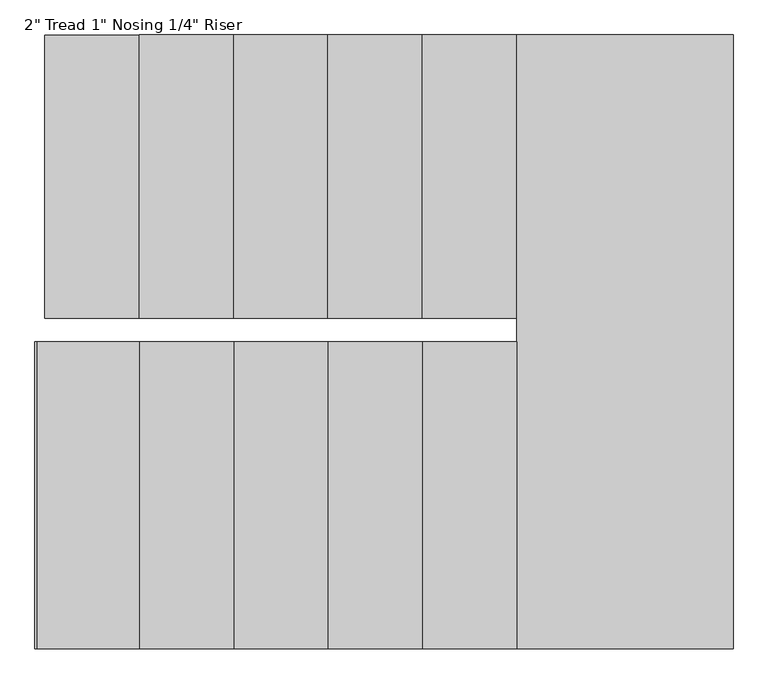
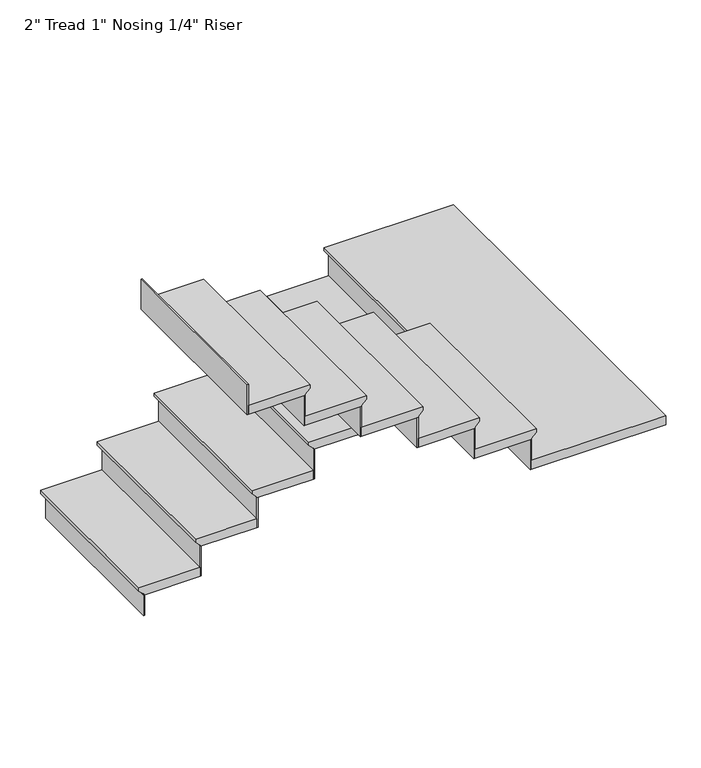
"""IFC4 building model written with IfcOpenShell, lengths in millimetres: stair flight geometry."""

from ifc_helpers import new_model, si_unit, origin, place, context, project, spatial, faceted_brep, source, transform, mapped, element, save


def stair_flight_96a85028(model_context):
    return source(origin(), model_context, "Body", "Brep", [
        faceted_brep([(-1179.0415084, -2827.3064015, 3350.6833333), (-1179.0415084, -2827.3064015, 3369.7333333), (-1179.0415084, -1912.9064015, 3369.7333333), (-1179.0415084, -1912.9064015, 3350.6833333), (-1153.6415084, -2827.3064015, 3325.2833333), (-1153.6415084, -1912.9064015, 3325.2833333), (-848.8415084, -2827.3064015, 3369.7333333), (-848.8415084, -1912.9064015, 3369.7333333), (-1153.6415084, -1912.9064015, 3318.9333333), (-848.8415084, -1912.9064015, 3318.9333333), (-848.8415084, -2827.3064015, 3318.9333333), (-1153.6415084, -2827.3064015, 3318.9333333)], [[[0, 1, 2, 3]], [[4, 0, 3, 5]], [[2, 1, 6, 7]], [[8, 9, 10, 11]], [[2, 7, 9, 8, 5, 3]], [[8, 11, 4, 5]], [[6, 1, 0, 4, 11, 10]], [[7, 6, 10, 9]]]),
        faceted_brep([(-1153.6415084, -2827.3064015, 3318.9333333), (-1153.6415084, -2827.3064015, 3200.4), (-1147.2915084, -2827.3064015, 3200.4), (-1147.2915084, -2827.3064015, 3318.9333333), (-1153.6415084, -1912.9064015, 3318.9333333), (-1147.2915084, -1912.9064015, 3318.9333333), (-1147.2915084, -1912.9064015, 3200.4), (-1153.6415084, -1912.9064015, 3200.4)], [[[0, 1, 2, 3]], [[4, 5, 6, 7]], [[1, 0, 4, 7]], [[2, 1, 7, 6]], [[3, 2, 6, 5]], [[0, 3, 5, 4]]]),
        faceted_brep([(-848.8415084, -2827.3064015, 3488.2666667), (-848.8415084, -2827.3064015, 3318.9333333), (-842.4915084, -2827.3064015, 3318.9333333), (-842.4915084, -2827.3064015, 3488.2666667), (-848.8415084, -1912.9064015, 3488.2666667), (-842.4915084, -1912.9064015, 3488.2666667), (-842.4915084, -1912.9064015, 3318.9333333), (-848.8415084, -1912.9064015, 3318.9333333)], [[[0, 1, 2, 3]], [[4, 5, 6, 7]], [[1, 0, 4, 7]], [[2, 1, 7, 6]], [[3, 2, 6, 5]], [[0, 3, 5, 4]]]),
        faceted_brep([(-874.2415084, -1912.9064015, 3539.0666667), (-874.2415084, -2827.3064015, 3539.0666667), (-544.0415084, -2827.3064015, 3539.0666667), (-544.0415084, -1912.9064015, 3539.0666667), (-848.8415084, -1912.9064015, 3488.2666667), (-544.0415084, -1912.9064015, 3488.2666667), (-544.0415084, -2827.3064015, 3488.2666667), (-848.8415084, -2827.3064015, 3488.2666667), (-848.8415084, -1912.9064015, 3494.6166667), (-874.2415084, -1912.9064015, 3520.0166667), (-848.8415084, -2827.3064015, 3494.6166667), (-874.2415084, -2827.3064015, 3520.0166667)], [[[0, 1, 2, 3]], [[4, 5, 6, 7]], [[0, 3, 5, 4, 8, 9]], [[4, 7, 10, 8]], [[2, 1, 11, 10, 7, 6]], [[3, 2, 6, 5]], [[11, 1, 0, 9]], [[10, 11, 9, 8]]]),
        faceted_brep([(-544.0415084, -2827.3064015, 3657.6), (-544.0415084, -2827.3064015, 3488.2666667), (-537.6915084, -2827.3064015, 3488.2666667), (-537.6915084, -2827.3064015, 3657.6), (-544.0415084, -1912.9064015, 3657.6), (-537.6915084, -1912.9064015, 3657.6), (-537.6915084, -1912.9064015, 3488.2666667), (-544.0415084, -1912.9064015, 3488.2666667)], [[[0, 1, 2, 3]], [[4, 5, 6, 7]], [[1, 0, 4, 7]], [[2, 1, 7, 6]], [[3, 2, 6, 5]], [[0, 3, 5, 4]]]),
        faceted_brep([(-569.4415084, -1912.9064015, 3708.4), (-569.4415084, -2827.3064015, 3708.4), (-239.2415084, -2827.3064015, 3708.4), (-239.2415084, -1912.9064015, 3708.4), (-544.0415084, -1912.9064015, 3657.6), (-239.2415084, -1912.9064015, 3657.6), (-239.2415084, -2827.3064015, 3657.6), (-544.0415084, -2827.3064015, 3657.6), (-544.0415084, -1912.9064015, 3663.95), (-569.4415084, -1912.9064015, 3689.35), (-544.0415084, -2827.3064015, 3663.95), (-569.4415084, -2827.3064015, 3689.35)], [[[0, 1, 2, 3]], [[4, 5, 6, 7]], [[0, 3, 5, 4, 8, 9]], [[4, 7, 10, 8]], [[2, 1, 11, 10, 7, 6]], [[3, 2, 6, 5]], [[11, 1, 0, 9]], [[10, 11, 9, 8]]]),
        faceted_brep([(-239.2415084, -2827.3064015, 3826.9333333), (-239.2415084, -2827.3064015, 3657.6), (-232.8915084, -2827.3064015, 3657.6), (-232.8915084, -2827.3064015, 3826.9333333), (-239.2415084, -1912.9064015, 3826.9333333), (-232.8915084, -1912.9064015, 3826.9333333), (-232.8915084, -1912.9064015, 3657.6), (-239.2415084, -1912.9064015, 3657.6)], [[[0, 1, 2, 3]], [[4, 5, 6, 7]], [[1, 0, 4, 7]], [[2, 1, 7, 6]], [[3, 2, 6, 5]], [[0, 3, 5, 4]]]),
        faceted_brep([(-264.6415084, -1912.9064015, 3877.7333333), (-264.6415084, -2827.3064015, 3877.7333333), (65.5584916, -2827.3064015, 3877.7333333), (65.5584916, -1912.9064015, 3877.7333333), (-239.2415084, -1912.9064015, 3826.9333333), (65.5584916, -1912.9064015, 3826.9333333), (65.5584916, -2827.3064015, 3826.9333333), (-239.2415084, -2827.3064015, 3826.9333333), (-239.2415084, -1912.9064015, 3833.2833333), (-264.6415084, -1912.9064015, 3858.6833333), (-239.2415084, -2827.3064015, 3833.2833333), (-264.6415084, -2827.3064015, 3858.6833333)], [[[0, 1, 2, 3]], [[4, 5, 6, 7]], [[0, 3, 5, 4, 8, 9]], [[4, 7, 10, 8]], [[2, 1, 11, 10, 7, 6]], [[3, 2, 6, 5]], [[11, 1, 0, 9]], [[10, 11, 9, 8]]]),
        faceted_brep([(65.5584916, -2827.3064015, 3996.2666667), (65.5584916, -2827.3064015, 3826.9333333), (71.9084916, -2827.3064015, 3826.9333333), (71.9084916, -2827.3064015, 3996.2666667), (65.5584916, -1912.9064015, 3996.2666667), (71.9084916, -1912.9064015, 3996.2666667), (71.9084916, -1912.9064015, 3826.9333333), (65.5584916, -1912.9064015, 3826.9333333)], [[[0, 1, 2, 3]], [[4, 5, 6, 7]], [[1, 0, 4, 7]], [[2, 1, 7, 6]], [[3, 2, 6, 5]], [[0, 3, 5, 4]]]),
        faceted_brep([(40.1584916, -1912.9064015, 4047.0666667), (40.1584916, -2827.3064015, 4047.0666667), (370.3584916, -2827.3064015, 4047.0666667), (370.3584916, -1912.9064015, 4047.0666667), (65.5584916, -1912.9064015, 3996.2666667), (370.3584916, -1912.9064015, 3996.2666667), (370.3584916, -2827.3064015, 3996.2666667), (65.5584916, -2827.3064015, 3996.2666667), (65.5584916, -1912.9064015, 4002.6166667), (40.1584916, -1912.9064015, 4028.0166667), (65.5584916, -2827.3064015, 4002.6166667), (40.1584916, -2827.3064015, 4028.0166667)], [[[0, 1, 2, 3]], [[4, 5, 6, 7]], [[0, 3, 5, 4, 8, 9]], [[4, 7, 10, 8]], [[2, 1, 11, 10, 7, 6]], [[3, 2, 6, 5]], [[11, 1, 0, 9]], [[10, 11, 9, 8]]]),
        faceted_brep([(370.3584916, -2827.3064015, 4165.6), (370.3584916, -2827.3064015, 3996.2666667), (376.7084916, -2827.3064015, 3996.2666667), (376.7084916, -2827.3064015, 4165.6), (370.3584916, -1912.9064015, 4165.6), (376.7084916, -1912.9064015, 4165.6), (376.7084916, -1912.9064015, 3996.2666667), (370.3584916, -1912.9064015, 3996.2666667)], [[[0, 1, 2, 3]], [[4, 5, 6, 7]], [[1, 0, 4, 7]], [[2, 1, 7, 6]], [[3, 2, 6, 5]], [[0, 3, 5, 4]]]),
        faceted_brep([(319.5584916, -3894.1064015, 4216.4), (1043.4584916, -3894.1064015, 4216.4), (1043.4584916, -1912.9064015, 4216.4), (344.9584916, -1912.9064015, 4216.4), (344.9584916, -2903.5064015, 4216.4), (319.5584916, -2903.5064015, 4216.4), (1043.4584916, -3894.1064015, 4165.6), (319.5584916, -3894.1064015, 4165.6), (319.5584916, -2903.5064015, 4165.6), (344.9584916, -2903.5064015, 4165.6), (344.9584916, -2827.3064015, 4165.6), (370.3584916, -2827.3064015, 4165.6), (370.3584916, -1912.9064015, 4165.6), (1043.4584916, -1912.9064015, 4165.6), (370.3584916, -1912.9064015, 4171.95), (344.9584916, -1912.9064015, 4197.35), (370.3584916, -2827.3064015, 4171.95), (344.9584916, -2827.3064015, 4197.35)], [[[0, 1, 2, 3, 4, 5]], [[6, 7, 8, 9, 10, 11, 12, 13]], [[1, 0, 7, 6]], [[2, 1, 6, 13]], [[3, 2, 13, 12, 14, 15]], [[12, 11, 16, 14]], [[11, 10, 17, 16]], [[4, 3, 15, 17, 10, 9]], [[5, 4, 9, 8]], [[0, 5, 8, 7]], [[15, 14, 16, 17]]]),
        faceted_brep([(319.5584916, -2903.5064015, 4334.9333333), (319.5584916, -2903.5064015, 4165.6), (313.2084916, -2903.5064015, 4165.6), (313.2084916, -2903.5064015, 4334.9333333), (319.5584916, -3894.1064015, 4334.9333333), (313.2084916, -3894.1064015, 4334.9333333), (313.2084916, -3894.1064015, 4165.6), (319.5584916, -3894.1064015, 4165.6)], [[[0, 1, 2, 3]], [[4, 5, 6, 7]], [[1, 0, 4, 7]], [[2, 1, 7, 6]], [[3, 2, 6, 5]], [[0, 3, 5, 4]]]),
        faceted_brep([(344.9584916, -3894.1064015, 4385.7333333), (344.9584916, -2903.5064015, 4385.7333333), (14.7584916, -2903.5064015, 4385.7333333), (14.7584916, -3894.1064015, 4385.7333333), (319.5584916, -3894.1064015, 4334.9333333), (14.7584916, -3894.1064015, 4334.9333333), (14.7584916, -2903.5064015, 4334.9333333), (319.5584916, -2903.5064015, 4334.9333333), (319.5584916, -3894.1064015, 4341.2833333), (344.9584916, -3894.1064015, 4366.6833333), (319.5584916, -2903.5064015, 4341.2833333), (344.9584916, -2903.5064015, 4366.6833333)], [[[0, 1, 2, 3]], [[4, 5, 6, 7]], [[0, 3, 5, 4, 8, 9]], [[4, 7, 10, 8]], [[2, 1, 11, 10, 7, 6]], [[3, 2, 6, 5]], [[11, 1, 0, 9]], [[10, 11, 9, 8]]]),
        faceted_brep([(14.7584916, -2903.5064015, 4504.2666667), (14.7584916, -2903.5064015, 4334.9333333), (8.4084916, -2903.5064015, 4334.9333333), (8.4084916, -2903.5064015, 4504.2666667), (14.7584916, -3894.1064015, 4504.2666667), (8.4084916, -3894.1064015, 4504.2666667), (8.4084916, -3894.1064015, 4334.9333333), (14.7584916, -3894.1064015, 4334.9333333)], [[[0, 1, 2, 3]], [[4, 5, 6, 7]], [[1, 0, 4, 7]], [[2, 1, 7, 6]], [[3, 2, 6, 5]], [[0, 3, 5, 4]]]),
        faceted_brep([(40.1584916, -3894.1064015, 4555.0666667), (40.1584916, -2903.5064015, 4555.0666667), (-290.0415084, -2903.5064015, 4555.0666667), (-290.0415084, -3894.1064015, 4555.0666667), (14.7584916, -3894.1064015, 4504.2666667), (-290.0415084, -3894.1064015, 4504.2666667), (-290.0415084, -2903.5064015, 4504.2666667), (14.7584916, -2903.5064015, 4504.2666667), (14.7584916, -3894.1064015, 4510.6166667), (40.1584916, -3894.1064015, 4536.0166667), (14.7584916, -2903.5064015, 4510.6166667), (40.1584916, -2903.5064015, 4536.0166667)], [[[0, 1, 2, 3]], [[4, 5, 6, 7]], [[0, 3, 5, 4, 8, 9]], [[4, 7, 10, 8]], [[2, 1, 11, 10, 7, 6]], [[3, 2, 6, 5]], [[11, 1, 0, 9]], [[10, 11, 9, 8]]]),
        faceted_brep([(-290.0415084, -2903.5064015, 4673.6), (-290.0415084, -2903.5064015, 4504.2666667), (-296.3915084, -2903.5064015, 4504.2666667), (-296.3915084, -2903.5064015, 4673.6), (-290.0415084, -3894.1064015, 4673.6), (-296.3915084, -3894.1064015, 4673.6), (-296.3915084, -3894.1064015, 4504.2666667), (-290.0415084, -3894.1064015, 4504.2666667)], [[[0, 1, 2, 3]], [[4, 5, 6, 7]], [[1, 0, 4, 7]], [[2, 1, 7, 6]], [[3, 2, 6, 5]], [[0, 3, 5, 4]]]),
        faceted_brep([(-264.6415084, -3894.1064015, 4724.4), (-264.6415084, -2903.5064015, 4724.4), (-594.8415084, -2903.5064015, 4724.4), (-594.8415084, -3894.1064015, 4724.4), (-290.0415084, -3894.1064015, 4673.6), (-594.8415084, -3894.1064015, 4673.6), (-594.8415084, -2903.5064015, 4673.6), (-290.0415084, -2903.5064015, 4673.6), (-290.0415084, -3894.1064015, 4679.95), (-264.6415084, -3894.1064015, 4705.35), (-290.0415084, -2903.5064015, 4679.95), (-264.6415084, -2903.5064015, 4705.35)], [[[0, 1, 2, 3]], [[4, 5, 6, 7]], [[0, 3, 5, 4, 8, 9]], [[4, 7, 10, 8]], [[2, 1, 11, 10, 7, 6]], [[3, 2, 6, 5]], [[11, 1, 0, 9]], [[10, 11, 9, 8]]]),
        faceted_brep([(-594.8415084, -2903.5064015, 4842.9333333), (-594.8415084, -2903.5064015, 4673.6), (-601.1915084, -2903.5064015, 4673.6), (-601.1915084, -2903.5064015, 4842.9333333), (-594.8415084, -3894.1064015, 4842.9333333), (-601.1915084, -3894.1064015, 4842.9333333), (-601.1915084, -3894.1064015, 4673.6), (-594.8415084, -3894.1064015, 4673.6)], [[[0, 1, 2, 3]], [[4, 5, 6, 7]], [[1, 0, 4, 7]], [[2, 1, 7, 6]], [[3, 2, 6, 5]], [[0, 3, 5, 4]]]),
        faceted_brep([(-569.4415084, -3894.1064015, 4893.7333333), (-569.4415084, -2903.5064015, 4893.7333333), (-899.6415084, -2903.5064015, 4893.7333333), (-899.6415084, -3894.1064015, 4893.7333333), (-594.8415084, -3894.1064015, 4842.9333333), (-899.6415084, -3894.1064015, 4842.9333333), (-899.6415084, -2903.5064015, 4842.9333333), (-594.8415084, -2903.5064015, 4842.9333333), (-594.8415084, -3894.1064015, 4849.2833333), (-569.4415084, -3894.1064015, 4874.6833333), (-594.8415084, -2903.5064015, 4849.2833333), (-569.4415084, -2903.5064015, 4874.6833333)], [[[0, 1, 2, 3]], [[4, 5, 6, 7]], [[0, 3, 5, 4, 8, 9]], [[4, 7, 10, 8]], [[2, 1, 11, 10, 7, 6]], [[3, 2, 6, 5]], [[11, 1, 0, 9]], [[10, 11, 9, 8]]]),
        faceted_brep([(-899.6415084, -2903.5064015, 5012.2666667), (-899.6415084, -2903.5064015, 4842.9333333), (-905.9915084, -2903.5064015, 4842.9333333), (-905.9915084, -2903.5064015, 5012.2666667), (-899.6415084, -3894.1064015, 5012.2666667), (-905.9915084, -3894.1064015, 5012.2666667), (-905.9915084, -3894.1064015, 4842.9333333), (-899.6415084, -3894.1064015, 4842.9333333)], [[[0, 1, 2, 3]], [[4, 5, 6, 7]], [[1, 0, 4, 7]], [[2, 1, 7, 6]], [[3, 2, 6, 5]], [[0, 3, 5, 4]]]),
        faceted_brep([(-1204.4415084, -2903.5064015, 5181.6), (-1204.4415084, -2903.5064015, 5012.2666667), (-1210.7915084, -2903.5064015, 5012.2666667), (-1210.7915084, -2903.5064015, 5181.6), (-1204.4415084, -3894.1064015, 5181.6), (-1210.7915084, -3894.1064015, 5181.6), (-1210.7915084, -3894.1064015, 5012.2666667), (-1204.4415084, -3894.1064015, 5012.2666667)], [[[0, 1, 2, 3]], [[4, 5, 6, 7]], [[1, 0, 4, 7]], [[2, 1, 7, 6]], [[3, 2, 6, 5]], [[0, 3, 5, 4]]]),
        faceted_brep([(-874.2415084, -3894.1064015, 5063.0666667), (-874.2415084, -2903.5064015, 5063.0666667), (-1204.4415084, -2903.5064015, 5063.0666667), (-1204.4415084, -3894.1064015, 5063.0666667), (-899.6415084, -3894.1064015, 5012.2666667), (-1204.4415084, -3894.1064015, 5012.2666667), (-1204.4415084, -2903.5064015, 5012.2666667), (-899.6415084, -2903.5064015, 5012.2666667), (-899.6415084, -3894.1064015, 5018.6166667), (-874.2415084, -3894.1064015, 5044.0166667), (-899.6415084, -2903.5064015, 5018.6166667), (-874.2415084, -2903.5064015, 5044.0166667)], [[[0, 1, 2, 3]], [[4, 5, 6, 7]], [[0, 3, 5, 4, 8, 9]], [[4, 7, 10, 8]], [[2, 1, 11, 10, 7, 6]], [[3, 2, 6, 5]], [[11, 1, 0, 9]], [[10, 11, 9, 8]]]),
    ])


if __name__ == "__main__":
    model = new_model("IFC4")
    model_context = context("Model", 3, world=origin())
    ifc_project = project(units=[si_unit("LENGTHUNIT", "METRE", prefix="MILLI")], contexts=[model_context])
    site = spatial("IfcSite", under=ifc_project)
    building = spatial("IfcBuilding", under=site)
    placement = place(None, origin())
    stair_flight_shape = stair_flight_96a85028(model_context)
    element("IfcStairFlight", 1, ObjectType="2\" Tread 1\" Nosing 1/4\" Riser", at=placement, inside=building, context=model_context, shape_type="MappedRepresentation", body=[
        mapped(stair_flight_shape, transform((0.0, 0.0, 0.0), x_axis=(1.0, 0.0, 0.0), y_axis=(0.0, 1.0, 0.0), z_axis=(0.0, 0.0, 1.0))),
    ])
    save(model, "model.ifc")
